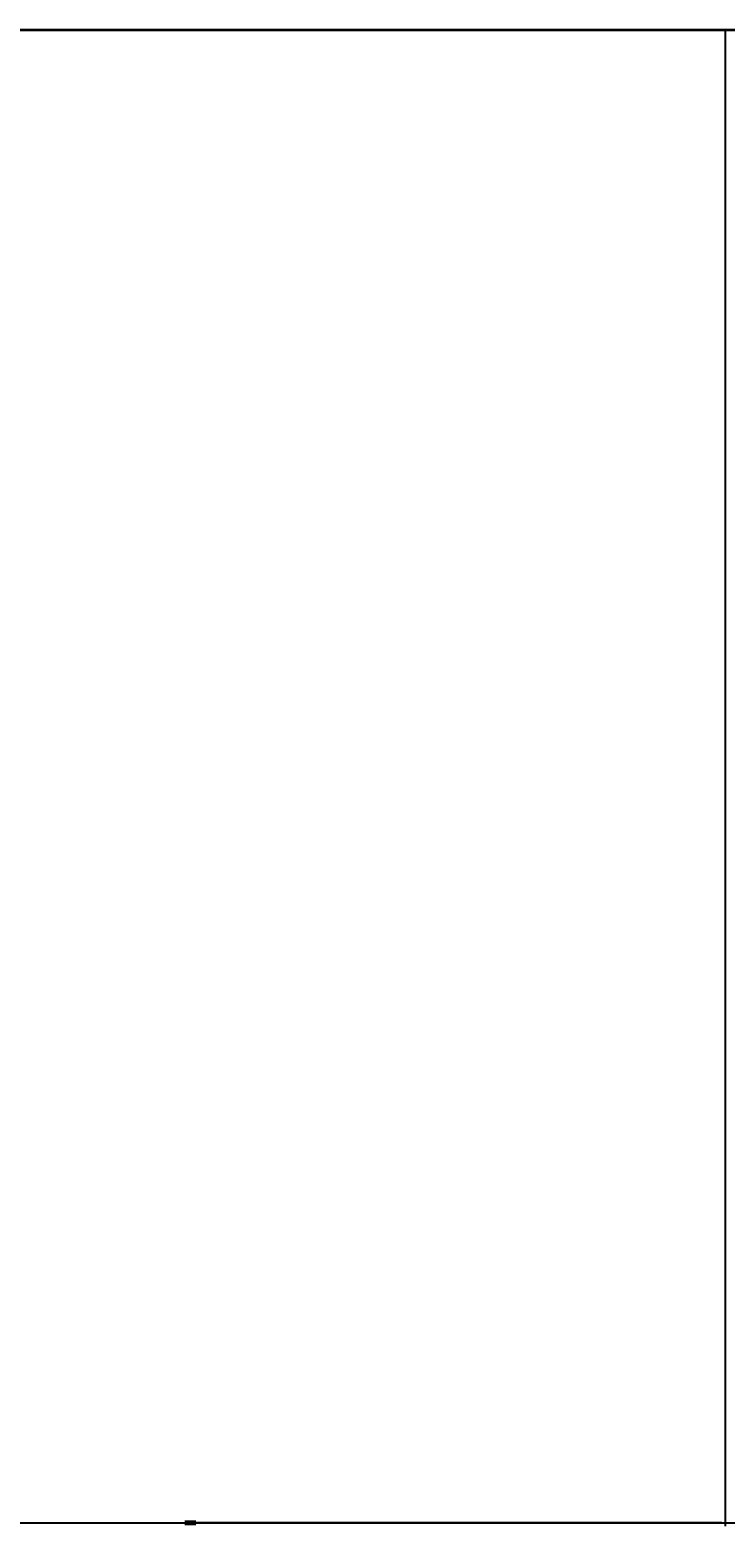
# Model space of a CAD drawing. Units: inches. Extents: x -128 to 854, y -395 to 398.
# Tile 9 of 61: x -16 to 23, y -382 to -298. Entities that reach past the tile are written whole.
import ezdxf

# ---------------------------------------------------------------- set-up
doc = ezdxf.new("R2010")
doc.units = ezdxf.units.IN
doc.header["$MEASUREMENT"] = 0
doc.layers.add('A-ANNO-DIMS', color=2, linetype='Continuous', lineweight=18)
doc.layers.add('A-SECT', color=220, linetype='Continuous', lineweight=35)
doc.styles.get("Standard").update_dxf_attribs({"font": 'arial.ttf'})
doc.dimstyles.get("Standard").update_dxf_attribs({"dimtxt": 0.18, "dimasz": 0.18, "dimexe": 0.18, "dimexo": 0.0625, "dimgap": 0.09, "dimtad": 0, "dimtih": 1, "dimtoh": 1, "dimdec": 1, "dimzin": 0, "dimdsep": 46, "dimlunit": 4, "dimtxsty": 'Standard', "dimcen": 0.09, "dimclrd": 1, "dimclre": 2, "dimclrt": 6, "dimadec": 0, "dimazin": 0, "dimtfac": 1, "dimtdec": 1, "dimtofl": 0, "dimtmove": 0, "dimatfit": 3, "dimfxl": 1, "dimtfill": 2, "dimtfillclr": 3, "dimtolj": 1, "dimtzin": 0, "dimarcsym": 0})

# ---------------------------------------------------------------- blocks, each defined once
blk = doc.blocks.new('*D123')
at = {"layer": 'A-ANNO-DIMS', "color": 2, "lineweight": -2, "transparency": 16777216}
for p, q in [((-17.161, -358.082), (-17.161, -381.899)), ((121.839, -358.082), (121.839, -381.899))]:
    blk.add_line(p, q, dxfattribs=at)
at = {"layer": 'A-ANNO-DIMS', "color": 1, "lineweight": -2, "transparency": 16777216}
for p, q in [((-16.981, -381.719), (51.948, -381.719)), ((121.659, -381.719), (52.73, -381.719))]:
    blk.add_line(p, q, dxfattribs=at)
at = {"layer": 'A-ANNO-DIMS', "color": 1, "transparency": 16777216}
for points in [[(-16.981, -381.689), (-16.981, -381.749), (-17.161, -381.719)], [(121.659, -381.689), (121.659, -381.749), (121.839, -381.719)]]:
    blk.add_solid(points, dxfattribs=at)
at = {"layer": 'Defpoints', "color": 0, "transparency": 16777216}
for p in [(-17.161, -358.019), (121.839, -358.019), (121.839, -381.719)]:
    blk.add_point(p, dxfattribs=at)
at = {"layer": 'A-ANNO-DIMS', "color": 6, "transparency": 16777216, "insert": (52.339, -381.719), "char_height": 0.18, "attachment_point": 5, "bg_fill": 1, "box_fill_scale": 1.25, "bg_fill_color": 3, "bg_fill_transparency": 0}
blk.add_mtext('\\A1;11\'-7"', dxfattribs=at)
blk = doc.blocks.new('*D125')
at = {"layer": 'A-ANNO-DIMS', "color": 2, "lineweight": -2, "transparency": 16777216}
for p, q in [((-37.161, -298.082), (-37.161, -381.899)), ((22.811, -298.082), (22.811, -381.899))]:
    blk.add_line(p, q, dxfattribs=at)
at = {"layer": 'A-ANNO-DIMS', "color": 1, "lineweight": -2, "transparency": 16777216}
for p, q in [((-36.981, -381.719), (-7.504, -381.719)), ((22.631, -381.719), (-6.846, -381.719))]:
    blk.add_line(p, q, dxfattribs=at)
at = {"layer": 'A-ANNO-DIMS', "color": 1, "transparency": 16777216}
for points in [[(-36.981, -381.689), (-36.981, -381.749), (-37.161, -381.719)], [(22.631, -381.689), (22.631, -381.749), (22.811, -381.719)]]:
    blk.add_solid(points, dxfattribs=at)
at = {"layer": 'Defpoints', "color": 0, "transparency": 16777216}
for p in [(-37.161, -298.019), (22.811, -298.019), (22.811, -381.719)]:
    blk.add_point(p, dxfattribs=at)
at = {"layer": 'A-ANNO-DIMS', "color": 6, "transparency": 16777216, "insert": (-7.175, -381.719), "char_height": 0.18, "attachment_point": 5, "bg_fill": 1, "box_fill_scale": 1.25, "bg_fill_color": 3, "bg_fill_transparency": 0}
blk.add_mtext('\\A1;5\'-0"', dxfattribs=at)

msp = doc.modelspace()

# ---------------------------------------------------------------- linework, layer by layer
at = {"layer": 'A-SECT'}
msp.add_line((-56.161, -298.019), (312.839, -298.019), dxfattribs=at)

# ---------------------------------------------------------------- dimensions: what is measured, and where the dimension line sits
at = {"layer": 'A-ANNO-DIMS'}
for base, p1, p2, picture, middle in [((22.811, -381.719), (-37.161, -298.019), (22.811, -298.019), '*D125', (-7.175, -381.719)), ((121.839, -381.719), (-17.161, -358.019), (121.839, -358.019), '*D123', (52.339, -381.719))]:
    dim = msp.add_linear_dim(base=base, p1=p1, p2=p2, dimstyle='Standard', override={"dimdec": 1, "dimlfac": 1, "dimrnd": 0, "dimzin": 1, "dimdsep": 46, "dimlunit": 4, "dimfrac": 2}, dxfattribs=at)
    dim.commit()
    dim.dimension.update_dxf_attribs({"geometry": picture, "text_midpoint": middle})

doc.saveas('drawing.dxf')
